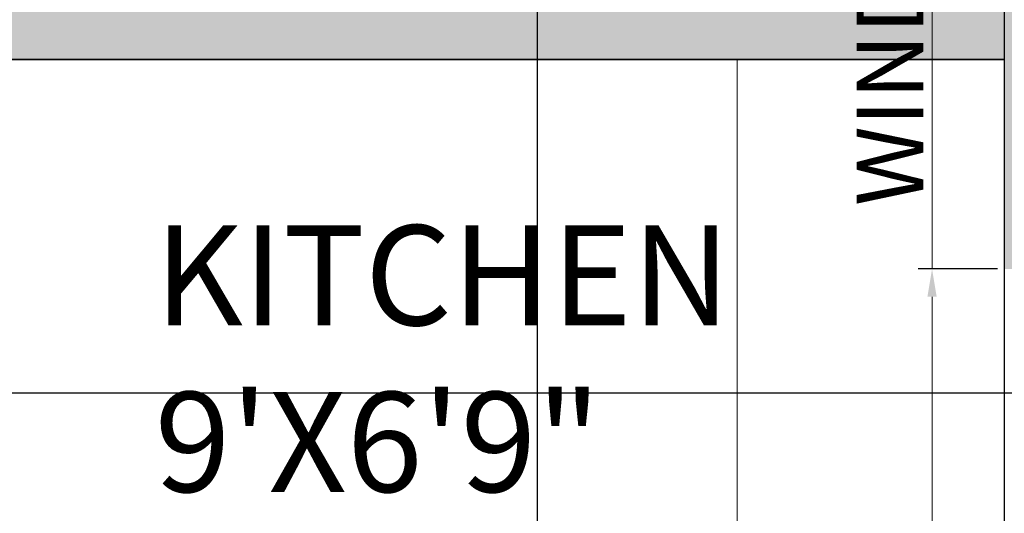
# Model space of a CAD drawing. Units: inches. Extents: x 2696 to 3240, y 1564 to 2310.
# Tile 27 of 76: x 3102 to 3191, y 1654 to 1699. Entities that reach past the tile are written whole.
import ezdxf

# ---------------------------------------------------------------- set-up
doc = ezdxf.new("R2010")
doc.units = ezdxf.units.IN
for name, color, linetype, lineweight in [('A-ANNO-DIMS', 3, 'Continuous', 18), ('A-AREA-IDEN', 7, 'Continuous', 18), ('A-FLOR-CASE', 8, 'Continuous', 18), ('A-WALL', 7, 'Continuous', 35), ('A-WALL-PATT', 9, 'Continuous', 13)]:
    doc.layers.add(name, color=color, linetype=linetype, lineweight=lineweight)
doc.styles.add('TIMES NEW', font='times.ttf')
doc.styles.add('YQ_DIM', font='SUPEROS.SHX', dxfattribs={"width": 0.8, "bigfont": 'HZDX.SHX'})
doc.dimstyles.new('Siddhuu', dxfattribs={"dimtxt": 6, "dimasz": 2.5, "dimexe": 1.25, "dimexo": 0.625, "dimtad": 1, "dimdec": 1, "dimlunit": 4, "dimtxsty": 'TIMES NEW', "dimcen": 2.5, "dimclrd": 256, "dimclre": 1, "dimclrt": 7, "dimadec": 0, "dimazin": 0, "dimtfac": 1, "dimtdec": 1, "dimtmove": 0, "dimatfit": 3, "dimfxl": 1, "dimtolj": 1, "dimlwd": -1, "dimarcsym": 0})

# ---------------------------------------------------------------- blocks, each defined once
blk = doc.blocks.new('*D26')
at = {"layer": 'A-ANNO-DIMS', "transparency": 16777216}
for p, q in [((3184.115, 1676.355), (3184.115, 1772.168)), ((3184.115, 1635.548), (3184.115, 1673.855))]:
    blk.add_line(p, q, dxfattribs=at)
at = {"layer": 'A-ANNO-DIMS', "color": 1, "lineweight": -2, "transparency": 16777216}
for p, q in [((3189.986, 1676.355), (3182.865, 1676.355)), ((3189.986, 1633.048), (3182.865, 1633.048))]:
    blk.add_line(p, q, dxfattribs=at)
at = {"layer": 'A-ANNO-DIMS', "transparency": 16777216}
for points in [[(3183.699, 1673.855), (3184.532, 1673.855), (3184.115, 1676.355)], [(3183.699, 1635.548), (3184.532, 1635.548), (3184.115, 1633.048)]]:
    blk.add_solid(points, dxfattribs=at)
at = {"layer": 'Defpoints', "color": 0, "transparency": 16777216}
for p in [(3184.115, 1676.355), (3190.611, 1676.355), (3190.611, 1633.048)]:
    blk.add_point(p, dxfattribs=at)
at = {"layer": 'A-ANNO-DIMS', "color": 7, "transparency": 16777216, "insert": (3180.348, 1725.511), "char_height": 6, "attachment_point": 5, "rotation": 90, "style": 'TIMES NEW'}
blk.add_mtext('\\A1;WINDOW 3\'-7 1/2" TYP.', dxfattribs=at)
blk = doc.blocks.new('*D51')
at = {"layer": 'A-ANNO-DIMS', "color": 1, "lineweight": -2, "transparency": 16777216}
for p, q in [((3016.611, 1979.576), (3016.611, 1568.951)), ((3148.611, 1979.576), (3148.611, 1568.951))]:
    blk.add_line(p, q, dxfattribs=at)
at = {"layer": 'A-ANNO-DIMS', "transparency": 16777216}
blk.add_line((3019.111, 1570.201), (3146.111, 1570.201), dxfattribs=at)
for points in [[(3019.111, 1570.618), (3019.111, 1569.784), (3016.611, 1570.201)], [(3146.111, 1570.618), (3146.111, 1569.784), (3148.611, 1570.201)]]:
    blk.add_solid(points, dxfattribs=at)
at = {"layer": 'Defpoints', "color": 0, "transparency": 16777216}
for p in [(3016.611, 1980.201), (3148.611, 1980.201), (3148.611, 1570.201)]:
    blk.add_point(p, dxfattribs=at)
at = {"layer": 'A-ANNO-DIMS', "color": 7, "transparency": 16777216, "insert": (3082.611, 1573.878), "char_height": 6, "attachment_point": 5, "style": 'TIMES NEW'}
blk.add_mtext('\\A1;11\'-0"', dxfattribs=at)
blk = doc.blocks.new('*D52')
at = {"layer": 'A-ANNO-DIMS', "color": 1, "lineweight": -2, "transparency": 16777216}
for p, q in [((3148.611, 1979.576), (3148.611, 1568.951)), ((3190.611, 1979.576), (3190.611, 1568.951))]:
    blk.add_line(p, q, dxfattribs=at)
at = {"layer": 'A-ANNO-DIMS', "transparency": 16777216}
blk.add_line((3151.111, 1570.201), (3188.111, 1570.201), dxfattribs=at)
for points in [[(3151.111, 1570.618), (3151.111, 1569.784), (3148.611, 1570.201)], [(3188.111, 1570.618), (3188.111, 1569.784), (3190.611, 1570.201)]]:
    blk.add_solid(points, dxfattribs=at)
at = {"layer": 'Defpoints', "color": 0, "transparency": 16777216}
for p in [(3148.611, 1980.201), (3190.611, 1980.201), (3190.611, 1570.201)]:
    blk.add_point(p, dxfattribs=at)
at = {"layer": 'A-ANNO-DIMS', "color": 7, "transparency": 16777216, "insert": (3169.611, 1573.878), "char_height": 6, "attachment_point": 5, "style": 'TIMES NEW'}
blk.add_mtext('\\A1;3\'-6"', dxfattribs=at)
blk = doc.blocks.new('*D56')
at = {"layer": 'A-ANNO-DIMS', "color": 1, "lineweight": -2, "transparency": 16777216}
for p, q in [((2966.334, 1884.201), (3235.861, 1884.201)), ((2966.334, 1665.201), (3235.861, 1665.201))]:
    blk.add_line(p, q, dxfattribs=at)
at = {"layer": 'A-ANNO-DIMS', "transparency": 16777216}
blk.add_line((3234.611, 1667.701), (3234.611, 1881.701), dxfattribs=at)
for points in [[(3234.195, 1881.701), (3235.028, 1881.701), (3234.611, 1884.201)], [(3234.195, 1667.701), (3235.028, 1667.701), (3234.611, 1665.201)]]:
    blk.add_solid(points, dxfattribs=at)
at = {"layer": 'Defpoints', "color": 0, "transparency": 16777216}
for p in [(2965.709, 1884.201), (3234.611, 1884.201), (2965.709, 1665.201)]:
    blk.add_point(p, dxfattribs=at)
at = {"layer": 'A-ANNO-DIMS', "color": 7, "transparency": 16777216, "insert": (3230.934, 1774.701), "char_height": 6, "attachment_point": 5, "rotation": 90, "style": 'TIMES NEW'}
blk.add_mtext('\\A1;18\'-3"', dxfattribs=at)

msp = doc.modelspace()

# ---------------------------------------------------------------- hatches: boundary and pattern name
at = {"layer": 'A-WALL-PATT', "transparency": 33554556}
h = msp.add_hatch(color=256, dxfattribs=at)
h.dxf.hatch_style = 1
h.paths.add_polyline_path([(2879.111, 2253.201), (2905.91, 2253.201), (2905.91, 2262.201), (2841.889, 2262.201), (2841.889, 2253.201), (2870.111, 2253.201), (2870.111, 2176.601), (2965.709, 2176.601), (2965.709, 2206.701), (2973.583, 2206.701), (2973.583, 2215.701), (2965.709, 2215.701), (2965.709, 2262.201), (2929.91, 2262.201), (2929.91, 2253.201), (2956.709, 2253.201), (2956.709, 2185.601), (2879.111, 2185.601)])
h.paths.add_polyline_path([(2782.834, 2262.201), (2745.611, 2262.201), (2745.611, 2228.729), (2754.611, 2228.729), (2754.611, 2253.201), (2782.834, 2253.201)])
h.paths.add_polyline_path([(2754.611, 2136.201), (2965.709, 2136.201), (2965.709, 2145.201), (2879.111, 2145.201), (2879.111, 2147.074), (2877.34, 2147.074), (2870.111, 2147.074), (2870.111, 2145.201), (2754.611, 2145.201), (2754.611, 2169.674), (2745.611, 2169.674), (2745.611, 2000.201), (2754.611, 2000.201), (2754.611, 2019.201), (2849.083, 2019.201), (2849.083, 2023.701), (2841.209, 2023.701), (2841.209, 2051.827), (2836.709, 2051.827), (2836.709, 2023.701), (2754.611, 2023.701), (2754.611, 2091.201), (2836.709, 2091.201), (2836.709, 2087.827), (2841.209, 2087.827), (2841.209, 2095.701), (2754.611, 2095.701)])
h.paths.add_polyline_path([(2965.709, 2136.201), (2956.709, 2136.201), (2956.709, 2023.701), (2885.083, 2023.701), (2885.083, 2019.201), (2956.709, 2019.201), (2956.709, 1950.575), (2965.709, 1950.575), (2965.709, 1980.201), (2973.583, 1980.201), (2973.583, 1989.201), (2965.709, 1989.201)])
h.paths.add_polyline_path([(2754.611, 1906.701), (2880.209, 1906.701), (2884.709, 1906.701), (2956.709, 1906.701), (2956.709, 1792.701), (2944.709, 1792.701), (2944.709, 1783.701), (2956.709, 1783.701), (2956.709, 1740.201), (2884.709, 1740.201), (2884.709, 1783.701), (2896.709, 1783.701), (2896.709, 1792.701), (2884.709, 1792.701), (2884.709, 1846.701), (2880.209, 1846.701), (2880.209, 1740.201), (2754.611, 1740.201), (2754.611, 1777.201), (2745.611, 1777.201), (2745.611, 1692.701), (2754.611, 1692.701), (2754.611, 1731.201), (2956.709, 1731.201), (2956.709, 1723.327), (2965.709, 1723.327), (2965.709, 1884.201), (2973.583, 1884.201), (2973.583, 1893.201), (2965.709, 1893.201), (2965.709, 1914.575), (2956.709, 1914.575), (2956.709, 1911.201), (2754.611, 1911.201), (2754.611, 1930.201), (2745.611, 1930.201), (2745.611, 1817.201), (2754.611, 1817.201), (2754.611, 1854.201), (2826.611, 1854.201), (2826.611, 1868.827), (2822.111, 1868.827), (2822.111, 1858.701), (2754.611, 1858.701)])
h.paths.add_polyline_path([(2965.709, 1656.201), (3008.237, 1656.201), (3008.237, 1665.201), (2965.709, 1665.201), (2965.709, 1693.327), (2956.709, 1693.327), (2956.709, 1686.201), (2934.583, 1686.201), (2934.583, 1681.701), (2956.709, 1681.701), (2956.709, 1614.201), (2896.709, 1614.201), (2896.709, 1681.701), (2904.583, 1681.701), (2904.583, 1686.201), (2892.209, 1686.201), (2892.209, 1614.201), (2858.41, 1614.201), (2858.41, 1605.201), (2965.709, 1605.201)])
h.paths.add_polyline_path([(2788.41, 1614.201), (2754.611, 1614.201), (2754.611, 1652.701), (2745.611, 1652.701), (2745.611, 1605.201), (2788.41, 1605.201)])
h.paths.add_polyline_path([(3199.611, 1633.048), (3190.611, 1633.048), (3190.611, 1614.201), (3082.611, 1614.201), (3082.611, 1665.201), (3070.237, 1665.201), (3070.237, 1656.201), (3078.111, 1656.201), (3078.111, 1605.201), (3199.611, 1605.201)])
h.paths.add_polyline_path([(3199.611, 1702.048), (3190.611, 1702.048), (3190.611, 1699.701), (3106.611, 1699.701), (3106.611, 1747.701), (3190.611, 1747.701), (3190.611, 1752.201), (3082.611, 1752.201), (3082.611, 1760.075), (3078.111, 1760.075), (3078.111, 1747.701), (3102.111, 1747.701), (3102.111, 1699.701), (3078.111, 1699.701), (3078.111, 1695.201), (3190.611, 1695.201), (3190.611, 1676.355), (3199.611, 1676.355)])
h.paths.add_polyline_path([(3199.611, 1783.201), (3190.611, 1783.201), (3190.611, 1745.355), (3199.611, 1745.355)])
h.paths.add_polyline_path([(3082.611, 1884.201), (3190.611, 1884.201), (3190.611, 1853.201), (3199.611, 1853.201), (3199.611, 1901.701), (3190.611, 1901.701), (3190.611, 1893.201), (3005.583, 1893.201), (3005.583, 1891.281), (3005.583, 1884.201), (3078.111, 1884.201), (3078.111, 1792.075), (3082.611, 1792.075)])
h.paths.add_polyline_path([(3199.611, 1994.701), (3190.611, 1994.701), (3190.611, 1989.201), (3073.709, 1989.201), (3073.709, 2034.201), (3069.209, 2034.201), (3069.209, 1989.201), (3005.583, 1989.201), (3005.583, 1980.201), (3190.611, 1980.201), (3190.611, 1971.701), (3199.611, 1971.701)])
h.paths.add_polyline_path([(3199.611, 2155.201), (3190.611, 2155.201), (3190.611, 2064.701), (3199.611, 2064.701)])
h.paths.add_polyline_path([(3190.611, 2074.701), (3106.611, 2074.701), (3106.611, 2122.701), (3190.611, 2122.701), (3190.611, 2127.201), (3082.709, 2127.201), (3082.709, 2135.075), (3073.709, 2135.075), (3073.709, 2122.701), (3102.111, 2122.701), (3102.111, 2074.701), (3069.209, 2074.701), (3069.209, 2070.201), (3190.611, 2070.201)])
h.paths.add_polyline_path([(3082.709, 2253.201), (3190.611, 2253.201), (3190.611, 2225.201), (3199.611, 2225.201), (3199.611, 2262.201), (3073.709, 2262.201), (3073.709, 2215.701), (3035.583, 2215.701), (3035.583, 2206.701), (3073.709, 2206.701), (3073.709, 2171.075), (3082.709, 2171.075)])

# ---------------------------------------------------------------- linework, layer by layer
at = {"layer": 'A-FLOR-CASE'}
msp.add_line((3166.611, 1638.201), (3166.611, 1695.201), dxfattribs=at)
at = {"layer": 'A-WALL'}
msp.add_line((3078.111, 1695.201), (3190.611, 1695.201), dxfattribs=at)

# ---------------------------------------------------------------- texts
at = {"layer": 'A-AREA-IDEN', "insert": (3114.246, 1680.292), "char_height": 9, "attachment_point": 1, "style": 'YQ_DIM'}
msp.add_mtext_dynamic_manual_height_columns('KITCHEN\\P9\'X6\'9"', width=48.00324, gutter_width=12.5, heights=[0], dxfattribs=at)

# ---------------------------------------------------------------- dimensions: what is measured, and where the dimension line sits
at = {"layer": 'A-ANNO-DIMS'}
for base, p1, p2, picture, middle in [((3148.611, 1570.201), (3016.611, 1980.201), (3148.611, 1980.201), '*D51', (3082.611, 1573.878)), ((3190.611, 1570.201), (3148.611, 1980.201), (3190.611, 1980.201), '*D52', (3169.611, 1573.878))]:
    dim = msp.add_linear_dim(base=base, p1=p1, p2=p2, dimstyle='Siddhuu', override={"dimdec": 1, "dimlfac": 1, "dimrnd": 0, "dimzin": 1, "dimdsep": 46, "dimlunit": 4, "dimfrac": 2}, dxfattribs=at)
    dim.commit()
    dim.dimension.update_dxf_attribs({"geometry": picture, "text_midpoint": middle})
dim = msp.add_linear_dim(base=(3234.611, 1884.201), p1=(2965.709, 1665.201), p2=(2965.709, 1884.201), angle=90, dimstyle='Siddhuu', override={"dimdec": 1, "dimlfac": 1, "dimrnd": 0, "dimzin": 1, "dimdsep": 46, "dimlunit": 4, "dimfrac": 2}, dxfattribs=at)
dim.commit()
dim.dimension.update_dxf_attribs({"geometry": '*D56', "text_midpoint": (3230.934, 1774.701)})
dim = msp.add_linear_dim(base=(3184.115, 1676.355), p1=(3190.611, 1633.048), p2=(3190.611, 1676.355), angle=90, text='WINDOW <> TYP.', dimstyle='Siddhuu', override={"dimdec": 1, "dimlfac": 1, "dimrnd": 0, "dimzin": 1, "dimdsep": 46, "dimlunit": 4, "dimfrac": 2}, dxfattribs=at)
dim.commit()
dim.dimension.update_dxf_attribs({"geometry": '*D26', "text_midpoint": (3180.348, 1725.511)})

doc.saveas('drawing.dxf')
